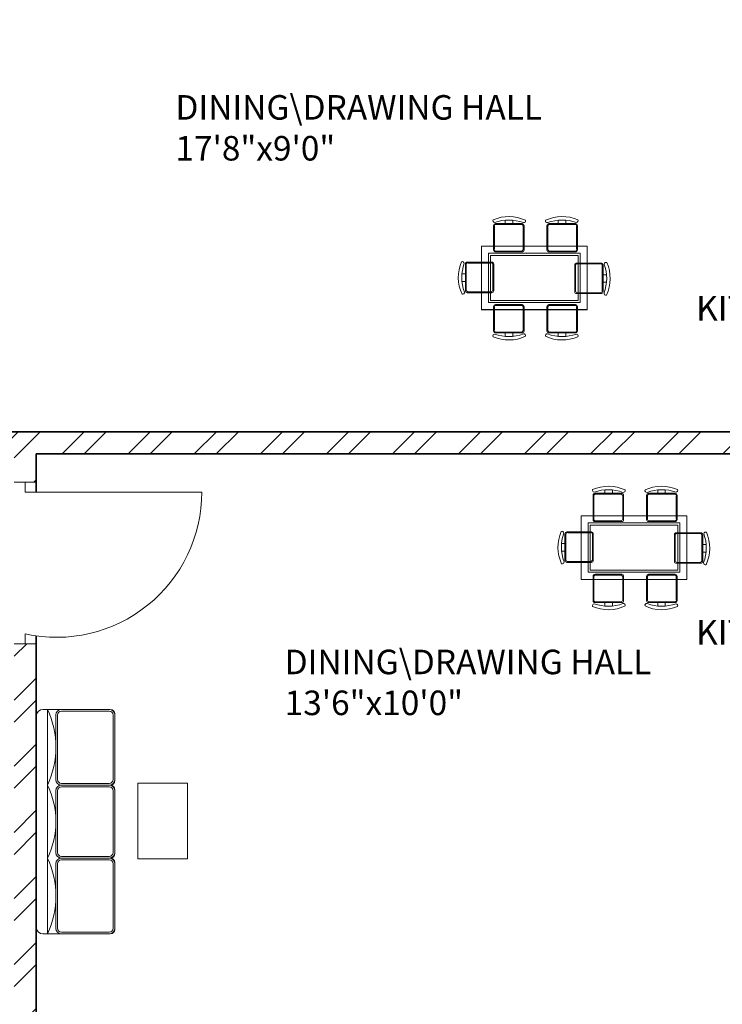
# Model space of a CAD drawing. Units: inches. Extents: x 2165 to 3042, y 1626 to 2968.
# Tile 7 of 11: x 2633 to 2776, y 1990 to 2191. Entities that reach past the tile are written whole.
import ezdxf

# ---------------------------------------------------------------- set-up
doc = ezdxf.new("R2010")
doc.units = ezdxf.units.IN
for name, color, linetype, lineweight in [('A-AREA-IDEN', 7, 'Continuous', 18), ('A-DOOR', 3, 'Continuous', 18), ('A-FURN', 8, 'Continuous', 13), ('A-WALL', 7, 'Continuous', 35), ('A-WALL-PATT', 252, 'Continuous', 13)]:
    doc.layers.add(name, color=color, linetype=linetype, lineweight=lineweight)
doc.styles.get("Standard").update_dxf_attribs({"font": 'arial.ttf'})

# ---------------------------------------------------------------- blocks, each defined once
blk = doc.blocks.new('TABLE-COFFEE')
blk.add_lwpolyline([(0, 15.45), (10.17, 15.45), (10.17, 0), (0, 0)], close=True)
blk = doc.blocks.new('DOOR-36-ENTRY')
for p, q in [((38.25, 32.9), (33.75, 32.9)), ((36, 32.9), (36, 30.9)), ((36, 30.9), (0, 30.9)), ((33.75, 0), (38.25, 0)), ((36, 0), (36, 2))]:
    blk.add_line(p, q)
blk.add_arc((29.6, 30.9), 29.6, 180, 282.4902)

msp = doc.modelspace()

# ---------------------------------------------------------------- hatches: boundary and pattern name
at = {"layer": 'A-WALL-PATT'}
h = msp.add_hatch(dxfattribs=at)
h.set_pattern_fill('ANSI32', color=256)
h.paths.add_polyline_path([(2406.4931, 2332.0783), (2286.6045, 2332.0783), (2286.6045, 2310.967), (2288.8545, 2310.967), (2291.1045, 2310.967), (2291.1045, 2327.5783), (2406.4931, 2327.5783), (2406.4931, 2329.8283)])
h.paths.add_polyline_path([(2439.6045, 2327.5783), (2444.9584, 2327.5783), (2444.9584, 2332.0783), (2430.2901, 2332.0783), (2430.2901, 2329.8283), (2430.2901, 2327.5783), (2435.1045, 2327.5783), (2435.1045, 2219.5783), (2431.0902, 2219.5783), (2431.0902, 2215.0783), (2435.1045, 2215.0783), (2444.1108, 2215.0783), (2444.1108, 2217.3283), (2444.1108, 2219.5783), (2439.6045, 2219.5783)])
h.paths.add_polyline_path([(2497.5418, 2329.8283), (2497.5418, 2332.0783), (2470.1978, 2332.0783), (2470.1978, 2327.5783), (2497.5418, 2327.5783)])
h.paths.add_polyline_path([(2617.9543, 2332.0783), (2557.5418, 2332.0783), (2557.5418, 2327.5783), (2583.6045, 2327.5783), (2583.6045, 2219.5783), (2474.0523, 2219.5783), (2474.0523, 2215.0783), (2583.6045, 2215.0783), (2583.6045, 2107.0783), (2579.3609, 2107.0783), (2579.3609, 2102.5783), (2588.1045, 2102.5783), (2593.5283, 2102.5783), (2593.5283, 2104.8283), (2593.5283, 2107.0783), (2588.1045, 2107.0783), (2588.1045, 2215.0783), (2691.2325, 2215.0783), (2691.2325, 2217.3283), (2691.2325, 2219.5783), (2588.1045, 2219.5783), (2588.1045, 2327.5783), (2617.9543, 2327.5783)])
h.paths.add_polyline_path([(2702.4444, 2329.8283), (2702.4444, 2332.0783), (2677.9543, 2332.0783), (2677.9543, 2327.5783), (2702.4444, 2327.5783)])
h.paths.add_polyline_path([(2736.6045, 2327.5783), (2742.5161, 2327.5783), (2742.5161, 2329.8283), (2742.5161, 2332.0783), (2727.7639, 2332.0783), (2727.7639, 2329.8283), (2727.7639, 2327.5783), (2732.1045, 2327.5783), (2732.1045, 2219.5783), (2726.4404, 2219.5783), (2726.4404, 2215.0783), (2732.1045, 2215.0783), (2742.7291, 2215.0783), (2742.7291, 2217.3283), (2742.7291, 2219.5783), (2736.6045, 2219.5783)])
h.paths.add_polyline_path([(2885.1045, 2332.0783), (2768.4887, 2332.0783), (2768.4887, 2327.5783), (2784.6045, 2327.5783), (2880.6045, 2327.5783), (2880.6045, 2310.967), (2885.1045, 2310.967)])
h.paths.add_polyline_path([(2885.1045, 2250.967), (2880.6045, 2250.967), (2880.6045, 2219.5783), (2776.5755, 2219.5783), (2776.5755, 2215.0783), (2788.1045, 2215.0783), (2788.1045, 2209.8634), (2790.3545, 2209.8634), (2792.6045, 2209.8634), (2792.6045, 2215.0783), (2880.6045, 2215.0783), (2880.6045, 2139.0783), (2871.2037, 2139.0783), (2871.2037, 2134.5783), (2885.1045, 2134.5783)])
h.paths.add_polyline_path([(2545.013, 2107.0783), (2474.0523, 2107.0783), (2291.1045, 2107.0783), (2291.1045, 2102.5783), (2535.6045, 2102.5783), (2535.6045, 2096.8046), (2537.8545, 2096.8046), (2540.1045, 2096.8046), (2540.1045, 2102.5783), (2545.013, 2102.5783), (2545.013, 2104.8283)])
h.paths.add_polyline_path([(2397.7297, 2217.3283), (2397.7297, 2219.5783), (2291.1045, 2219.5783), (2291.1045, 2250.967), (2286.6045, 2250.967), (2286.6045, 2206.1346), (2288.8545, 2206.1346), (2291.1045, 2206.1346), (2291.1045, 2215.0783), (2367.1045, 2215.0783), (2367.1045, 2212.2868), (2371.6045, 2212.2868), (2371.6045, 2215.0783), (2397.7297, 2215.0783)])
h.paths.add_polyline_path([(2291.1045, 1978.5783), (2367.1045, 1978.5783), (2371.6045, 1978.5783), (2373.2641, 1978.5783), (2374.4883, 1978.5783), (2374.4883, 1980.8283), (2374.4883, 1983.0783), (2371.6045, 1983.0783), (2371.6045, 1986.964), (2369.9051, 1986.964), (2369.3545, 1986.964), (2367.1045, 1986.964), (2367.1045, 1983.0783), (2291.1045, 1983.0783), (2291.1045, 2001.1808), (2286.6045, 2001.1808), (2286.6045, 1947.0203), (2288.8545, 1947.0203), (2291.1045, 1947.0203)])
h.paths.add_polyline_path([(2291.1045, 1887.0203), (2286.6045, 1887.0203), (2286.6045, 1842.0783), (2381.2561, 1842.0783), (2381.2561, 1844.3283), (2381.2561, 1846.5783), (2363.1045, 1846.5783), (2291.1045, 1846.5783)])
h.paths.add_polyline_path([(2415.6045, 1978.5783), (2421.1681, 1978.5783), (2421.1681, 1983.0783), (2415.6045, 1983.0783), (2406.5227, 1983.0783), (2406.5227, 1980.8283), (2406.5227, 1978.5783), (2411.1045, 1978.5783), (2411.1045, 1846.5783), (2406.7549, 1846.5783), (2406.7549, 1842.0783), (2419.2885, 1842.0783), (2419.2885, 1844.3283), (2419.2885, 1846.5783), (2415.6045, 1846.5783)])
h.paths.add_polyline_path([(2586.6045, 1982.779), (2586.6045, 1991.5911), (2582.1045, 1991.5911), (2582.1045, 1982.779), (2540.1045, 1982.779), (2540.1045, 2036.779), (2582.1045, 2036.779), (2582.1045, 2027.6051), (2586.6045, 2027.6051), (2586.6045, 2041.279), (2582.1045, 2041.279), (2540.1045, 2041.279), (2540.1045, 2063.9064), (2537.8545, 2063.9064), (2535.6045, 2063.9064), (2535.6045, 1983.0783), (2455.068, 1983.0783), (2455.068, 1978.5783), (2535.6045, 1978.5783), (2535.6045, 1846.5783), (2522.622, 1846.5783), (2522.622, 1842.0783), (2535.6045, 1842.0783), (2535.6045, 1806.0783), (2535.6045, 1801.5783), (2556.726, 1801.5783), (2556.726, 1803.8283), (2556.726, 1806.0783), (2540.1045, 1806.0783), (2540.1045, 1842.0783), (2540.1045, 1846.5783), (2540.1045, 1978.279), (2586.6045, 1978.279)])
h.paths.add_polyline_path([(2636.1045, 1978.5783), (2717.6642, 1978.5783), (2717.6642, 1980.8283), (2717.6642, 1983.0783), (2636.1045, 1983.0783), (2636.1045, 2063.9064), (2633.8545, 2063.9064), (2631.6045, 2063.9064), (2631.6045, 1846.5783), (2631.6045, 1842.0783), (2631.6045, 1806.0783), (2604.726, 1806.0783), (2604.726, 1801.5783), (2636.1045, 1801.5783), (2636.1045, 1842.0783), (2644.3411, 1842.0783), (2644.3411, 1844.3283), (2644.3411, 1846.5783), (2636.1045, 1846.5783)])
h.paths.add_polyline_path([(2760.6045, 1978.5783), (2764.9931, 1978.5783), (2764.9931, 1983.0783), (2750.4727, 1983.0783), (2750.4727, 1980.8283), (2750.4727, 1978.5783), (2756.1045, 1978.5783), (2756.1045, 1846.5783), (2749.4543, 1846.5783), (2749.4543, 1842.0783), (2765.1894, 1842.0783), (2765.1894, 1846.5783), (2760.6045, 1846.5783)])
h.paths.add_polyline_path([(2880.6045, 1983.0783), (2804.6045, 1983.0783), (2804.6045, 1988.3825), (2802.3545, 1988.3825), (2800.1045, 1988.3825), (2800.1045, 1983.0783), (2800.1045, 1978.5783), (2880.6045, 1978.5783)])
h.paths.add_polyline_path([(2885.1045, 2075.5783), (2871.2037, 2075.5783), (2871.2037, 2071.0783), (2880.6045, 2071.0783), (2880.6045, 1948.8144), (2885.1045, 1948.8144)])
h.paths.add_polyline_path([(2885.1045, 1888.8144), (2880.6045, 1888.8144), (2880.6045, 1846.5783), (2792.1167, 1846.5783), (2792.1167, 1842.0783), (2885.1045, 1842.0783)])
h.paths.add_polyline_path([(2724.4848, 1846.5783), (2708.1045, 1846.5783), (2692.3411, 1846.5783), (2692.3411, 1842.0783), (2724.4848, 1842.0783), (2724.4848, 1844.3283)])
h.paths.add_polyline_path([(2474.622, 1844.4672), (2474.622, 1846.5783), (2444.7417, 1846.5783), (2444.7417, 1842.0783), (2474.622, 1842.0783)])
h = msp.add_hatch(dxfattribs=at)
h.set_pattern_fill('ANSI32', color=256)
h.paths.add_polyline_path([(2834.3545, 2109.2607), (2832.1045, 2109.2607), (2829.8545, 2109.2607), (2829.8545, 2107.0783), (2788.1045, 2107.0783), (2627.8367, 2107.0783), (2627.8367, 2102.5783), (2631.6045, 2102.5783), (2631.6045, 2096.8046), (2636.1045, 2096.8046), (2636.1045, 2102.5783), (2788.1045, 2102.5783), (2829.8545, 2102.5783), (2829.8545, 2099.5599), (2834.3545, 2099.5599), (2834.3545, 2102.5783)])
h.paths.add_polyline_path([(2834.3545, 2162.7002), (2834.3545, 2167.2002), (2792.6045, 2167.2002), (2792.6045, 2188.8893), (2790.3545, 2188.8893), (2788.1045, 2188.8893), (2788.1045, 2162.7002), (2829.8545, 2162.7002), (2829.8545, 2134.5783), (2829.8545, 2129.9534), (2834.3545, 2129.9534), (2834.3545, 2134.5783), (2847.2037, 2134.5783), (2847.2037, 2139.0783), (2834.3545, 2139.0783)])
h.paths.add_polyline_path([(2834.3545, 2071.0783), (2847.2037, 2071.0783), (2847.2037, 2075.5783), (2834.3545, 2075.5783), (2834.3545, 2078.8214), (2829.8545, 2078.8214), (2829.8545, 2075.5783), (2829.8545, 2034.1177), (2800.1045, 2034.1177), (2800.1045, 2011.8162), (2802.3375, 2011.8162), (2804.6045, 2011.8162), (2804.6045, 2029.6177), (2834.3545, 2029.6177), (2834.3545, 2034.1177)])

# ---------------------------------------------------------------- linework, layer by layer
at = {"layer": 'A-DOOR'}
for p, q in [((2636.1045, 2096.8046), (2633.8545, 2096.8046)), ((2636.1045, 2063.9064), (2633.8545, 2063.9064))]:
    msp.add_line(p, q, dxfattribs=at)
at = {"layer": 'A-FURN'}
for points in [[(2729.5671, 2149.7833, -0.17580919), (2735.4417, 2149.7388, 0.57839206), (2735.8868, 2150.2282, 0.21452438), (2729.2556, 2150.3172, 0.55201397), (2729.5671, 2149.7833, -0.06507904)], [(2729.5672, 2149.7831, -0.17580919), (2735.4417, 2149.7386, 0.57839206), (2735.8868, 2150.228, 0.21452438), (2729.2556, 2150.3169, 0.55201397), (2729.5672, 2149.7831, -0.06507904)], [(2733.2769, 2149.5475), (2733.2769, 2150.2373, -0.06475861)], [(2733.2769, 2149.5473), (2733.2769, 2150.237, -0.06475861)], [(2740.3874, 2149.7388, -0.57839206), (2739.9423, 2150.2282, -0.21452438), (2746.5735, 2150.3172, -0.55201397), (2746.2619, 2149.7833, 0.1758092), (2740.3874, 2149.7388)], [(2740.3874, 2149.7386, -0.57839206), (2739.9423, 2150.228, -0.21452438), (2746.5735, 2150.3169, -0.55201397), (2746.2619, 2149.7831, 0.1758092), (2740.3874, 2149.7386)], [(2742.5522, 2149.5475), (2742.5522, 2150.2373, 0.06475861)], [(2742.5522, 2149.5473), (2742.5522, 2150.237, 0.06475861)], [(2735.1925, 2149.5475), (2729.7387, 2149.5475, 0.41421356), (2729.3572, 2149.166), (2729.3572, 2144.1514, 0.41421356), (2729.7387, 2143.7698), (2735.1925, 2143.7698, 0.41421356), (2735.574, 2144.1514), (2735.574, 2149.166, 0.41421356), (2735.1925, 2149.5475)], [(2735.1925, 2149.5473), (2729.7387, 2149.5473, 0.41421356), (2729.3572, 2149.1658), (2729.3572, 2144.1511, 0.41421356), (2729.7387, 2143.7696), (2735.1925, 2143.7696, 0.41421356), (2735.574, 2144.1511), (2735.574, 2149.1658, 0.41421356), (2735.1925, 2149.5473)], [(2746.0904, 2149.5475, -0.41421356), (2746.4719, 2149.166), (2746.4719, 2144.1514, -0.41421356), (2746.0904, 2143.7698), (2740.6366, 2143.7698, -0.41421356), (2740.255, 2144.1514), (2740.255, 2149.166, -0.41421356), (2740.6366, 2149.5475), (2746.0904, 2149.5475)], [(2746.0904, 2149.5473, -0.41421356), (2746.4719, 2149.1658), (2746.4719, 2144.1511, -0.41421356), (2746.0904, 2143.7696), (2740.6366, 2143.7696, -0.41421356), (2740.2551, 2144.1511), (2740.2551, 2149.1658, -0.41421356), (2740.6366, 2149.5473), (2746.0904, 2149.5473)], [(2723.4212, 2135.5971, -0.57839206), (2722.9318, 2135.152, -0.21452438), (2722.8429, 2141.7832, -0.55201397), (2723.3767, 2141.4717, 0.17580937), (2723.4212, 2135.5971)], [(2723.4212, 2135.5969, -0.57839206), (2722.9319, 2135.1518, -0.21452438), (2722.8429, 2141.783, -0.55201397), (2723.3767, 2141.4714, 0.17580937), (2723.4212, 2135.5969)], [(2723.6125, 2141.3001, -0.41421356), (2723.994, 2141.6816), (2729.0087, 2141.6816, -0.41421356), (2729.3902, 2141.3001), (2729.3902, 2135.8463, -0.41421356), (2729.0087, 2135.4648), (2723.994, 2135.4648, -0.41421356), (2723.6125, 2135.8463), (2723.6125, 2141.3001)], [(2723.6125, 2141.2999, -0.41421356), (2723.9941, 2141.6814), (2729.0087, 2141.6814, -0.41421356), (2729.3902, 2141.2999), (2729.3902, 2135.8461, -0.41421356), (2729.0087, 2135.4645), (2723.9941, 2135.4645, -0.41421356), (2723.6125, 2135.8461), (2723.6125, 2141.2999)], [(2751.6968, 2141.1133, 0.41421356), (2751.3153, 2141.4949), (2746.3006, 2141.4949, 0.41421356), (2745.9191, 2141.1133), (2745.9191, 2135.6595, 0.41421356), (2746.3006, 2135.278), (2751.3153, 2135.278, 0.41421356), (2751.6968, 2135.6595), (2751.6968, 2141.1133)], [(2751.6968, 2141.1131, 0.41421356), (2751.3153, 2141.4946), (2746.3006, 2141.4946, 0.41421356), (2745.9191, 2141.1131), (2745.9191, 2135.6593, 0.41421356), (2746.3006, 2135.2778), (2751.3153, 2135.2778, 0.41421356), (2751.6968, 2135.6593), (2751.6968, 2141.1131)], [(2751.9326, 2141.2849, -0.17580919), (2751.8881, 2135.4103, 0.57839206), (2752.3775, 2134.9653, 0.21452438), (2752.4664, 2141.5964, 0.55201397), (2751.9326, 2141.2849, -0.06507904)], [(2751.9326, 2141.2847, -0.17580919), (2751.8881, 2135.4101, 0.57839206), (2752.3775, 2134.965, 0.21452438), (2752.4664, 2141.5962, 0.55201397), (2751.9326, 2141.2847, -0.06507904)], [(2723.6125, 2137.762), (2722.9228, 2137.762, 0.06475861)], [(2723.6125, 2137.7617), (2722.9228, 2137.7617, 0.06475861)], [(2751.6968, 2137.5752), (2752.3865, 2137.5752, -0.06475861)], [(2751.6968, 2137.575), (2752.3866, 2137.575, -0.06475861)], [(2735.1925, 2127.2563), (2729.7387, 2127.2563, -0.41421356), (2729.3572, 2127.6378), (2729.3572, 2132.6525, -0.41421356), (2729.7387, 2133.034), (2735.1925, 2133.034, -0.41421356), (2735.574, 2132.6525), (2735.574, 2127.6378, -0.41421356), (2735.1925, 2127.2563)], [(2735.1925, 2127.2561), (2729.7387, 2127.2561, -0.41421356), (2729.3572, 2127.6376), (2729.3572, 2132.6522, -0.41421356), (2729.7387, 2133.0338), (2735.1925, 2133.0338, -0.41421356), (2735.574, 2132.6522), (2735.574, 2127.6376, -0.41421356), (2735.1925, 2127.2561)], [(2746.0904, 2127.2563, 0.41421356), (2746.4719, 2127.6378), (2746.4719, 2132.6525, 0.41421356), (2746.0904, 2133.034), (2740.6366, 2133.034, 0.41421356), (2740.255, 2132.6525), (2740.255, 2127.6378, 0.41421356), (2740.6366, 2127.2563), (2746.0904, 2127.2563)], [(2746.0904, 2127.2561, 0.41421356), (2746.4719, 2127.6376), (2746.4719, 2132.6522, 0.41421356), (2746.0904, 2133.0338), (2740.6366, 2133.0338, 0.41421356), (2740.2551, 2132.6522), (2740.2551, 2127.6376, 0.41421356), (2740.6366, 2127.2561), (2746.0904, 2127.2561)], [(2735.4417, 2127.065, -0.57839206), (2735.8868, 2126.5756, -0.21452438), (2729.2556, 2126.4867, -0.55201397), (2729.5671, 2127.0205, 0.17580929), (2735.4417, 2127.065)], [(2735.4417, 2127.0648, -0.57839206), (2735.8868, 2126.5754, -0.21452438), (2729.2556, 2126.4864, -0.55201397), (2729.5672, 2127.0203, 0.17580929), (2735.4417, 2127.0648)], [(2733.2769, 2127.2563), (2733.2769, 2126.5666, 0.06475861)], [(2733.2769, 2127.2561), (2733.2769, 2126.5663, 0.06475861)], [(2746.2619, 2127.0205, -0.17580928), (2740.3874, 2127.065, 0.57839206), (2739.9423, 2126.5756, 0.21452438), (2746.5735, 2126.4867, 0.55201397), (2746.2619, 2127.0205, -0.06507904)], [(2746.2619, 2127.0203, -0.17580928), (2740.3874, 2127.0648, 0.57839206), (2739.9423, 2126.5754, 0.21452438), (2746.5735, 2126.4864, 0.55201397), (2746.2619, 2127.0203, -0.06507904)], [(2742.5522, 2127.2563), (2742.5522, 2126.5666, -0.06475861)], [(2742.5522, 2127.2561), (2742.5522, 2126.5663, -0.06475861)], [(2749.8774, 2094.8015, -0.17580919), (2755.752, 2094.757, 0.57839206), (2756.197, 2095.2464, 0.21452438), (2749.5659, 2095.3354, 0.55201397), (2749.8774, 2094.8015, -0.06507904)], [(2749.8774, 2094.8013, -0.17580919), (2755.752, 2094.7568, 0.57839206), (2756.197, 2095.2462, 0.21452438), (2749.5659, 2095.3351, 0.55201397), (2749.8774, 2094.8013, -0.06507904)], [(2760.6976, 2094.757, -0.57839206), (2760.2526, 2095.2464, -0.21452438), (2766.8837, 2095.3354, -0.55201397), (2766.5722, 2094.8015, 0.1758092), (2760.6976, 2094.757)], [(2760.6976, 2094.7568, -0.57839206), (2760.2526, 2095.2462, -0.21452438), (2766.8837, 2095.3351, -0.55201397), (2766.5722, 2094.8013, 0.1758092), (2760.6976, 2094.7568)], [(2755.5027, 2094.5657), (2750.049, 2094.5657, 0.41421356), (2749.6674, 2094.1842), (2749.6674, 2089.1696, 0.41421356), (2750.049, 2088.788), (2755.5027, 2088.788, 0.41421356), (2755.8843, 2089.1696), (2755.8843, 2094.1842, 0.41421356), (2755.5027, 2094.5657)], [(2755.5027, 2094.5655), (2750.049, 2094.5655, 0.41421356), (2749.6674, 2094.184), (2749.6674, 2089.1693, 0.41421356), (2750.049, 2088.7878), (2755.5027, 2088.7878, 0.41421356), (2755.8843, 2089.1693), (2755.8843, 2094.184, 0.41421356), (2755.5027, 2094.5655)], [(2753.5871, 2094.5657), (2753.5871, 2095.2555, -0.06475861)], [(2753.5871, 2094.5655), (2753.5871, 2095.2553, -0.06475861)], [(2766.4006, 2094.5657, -0.41421356), (2766.7821, 2094.1842), (2766.7821, 2089.1696, -0.41421356), (2766.4006, 2088.788), (2760.9468, 2088.788, -0.41421356), (2760.5653, 2089.1696), (2760.5653, 2094.1842, -0.41421356), (2760.9468, 2094.5657), (2766.4006, 2094.5657)], [(2766.4006, 2094.5655, -0.41421356), (2766.7822, 2094.184), (2766.7822, 2089.1693, -0.41421356), (2766.4006, 2088.7878), (2760.9468, 2088.7878, -0.41421356), (2760.5653, 2089.1693), (2760.5653, 2094.184, -0.41421356), (2760.9468, 2094.5655), (2766.4006, 2094.5655)], [(2762.8625, 2094.5657), (2762.8625, 2095.2555, 0.06475861)], [(2762.8625, 2094.5655), (2762.8625, 2095.2553, 0.06475861)], [(2743.7314, 2080.6153, -0.57839206), (2743.2421, 2080.1703, -0.21452438), (2743.1531, 2086.8014, -0.55201397), (2743.687, 2086.4899, 0.17580937), (2743.7314, 2080.6153)], [(2743.7315, 2080.6151, -0.57839206), (2743.2421, 2080.17, -0.21452438), (2743.1531, 2086.8012, -0.55201397), (2743.687, 2086.4897, 0.17580937), (2743.7315, 2080.6151)], [(2743.9227, 2086.3183, -0.41421356), (2744.3043, 2086.6999), (2749.3189, 2086.6999, -0.41421356), (2749.7005, 2086.3183), (2749.7005, 2080.8645, -0.41421356), (2749.3189, 2080.483), (2744.3043, 2080.483, -0.41421356), (2743.9227, 2080.8645), (2743.9227, 2086.3183)], [(2743.9228, 2086.3181, -0.41421356), (2744.3043, 2086.6996), (2749.3189, 2086.6996, -0.41421356), (2749.7005, 2086.3181), (2749.7005, 2080.8643, -0.41421356), (2749.3189, 2080.4828), (2744.3043, 2080.4828, -0.41421356), (2743.9228, 2080.8643), (2743.9228, 2086.3181)], [(2772.0071, 2086.1315, 0.41421356), (2771.6255, 2086.5131), (2766.6109, 2086.5131, 0.41421356), (2766.2293, 2086.1315), (2766.2293, 2080.6778, 0.41421356), (2766.6109, 2080.2962), (2771.6255, 2080.2962, 0.41421356), (2772.0071, 2080.6778), (2772.0071, 2086.1315)], [(2772.0071, 2086.1313, 0.41421356), (2771.6255, 2086.5128), (2766.6109, 2086.5128, 0.41421356), (2766.2293, 2086.1313), (2766.2293, 2080.6775, 0.41421356), (2766.6109, 2080.296), (2771.6255, 2080.296, 0.41421356), (2772.0071, 2080.6775), (2772.0071, 2086.1313)], [(2772.2428, 2086.3031, -0.17580919), (2772.1983, 2080.4285, 0.57839206), (2772.6877, 2079.9835, 0.21452438), (2772.7767, 2086.6146, 0.55201397), (2772.2428, 2086.3031, -0.06507904)], [(2772.2428, 2086.3029, -0.17580919), (2772.1984, 2080.4283, 0.57839206), (2772.6877, 2079.9833, 0.21452438), (2772.7767, 2086.6144, 0.55201397), (2772.2428, 2086.3029, -0.06507904)], [(2743.9227, 2082.7802), (2743.233, 2082.7802, 0.06475861)], [(2743.9228, 2082.7799), (2743.233, 2082.7799, 0.06475861)], [(2772.0071, 2082.5934), (2772.6968, 2082.5934, -0.06475861)], [(2772.0071, 2082.5932), (2772.6968, 2082.5932, -0.06475861)], [(2755.5027, 2072.2745), (2750.049, 2072.2745, -0.41421356), (2749.6674, 2072.6561), (2749.6674, 2077.6707, -0.41421356), (2750.049, 2078.0522), (2755.5027, 2078.0522, -0.41421356), (2755.8843, 2077.6707), (2755.8843, 2072.6561, -0.41421356), (2755.5027, 2072.2745)], [(2755.5027, 2072.2743), (2750.049, 2072.2743, -0.41421356), (2749.6674, 2072.6558), (2749.6674, 2077.6705, -0.41421356), (2750.049, 2078.052), (2755.5027, 2078.052, -0.41421356), (2755.8843, 2077.6705), (2755.8843, 2072.6558, -0.41421356), (2755.5027, 2072.2743)], [(2766.4006, 2072.2745, 0.41421356), (2766.7821, 2072.6561), (2766.7821, 2077.6707, 0.41421356), (2766.4006, 2078.0522), (2760.9468, 2078.0522, 0.41421356), (2760.5653, 2077.6707), (2760.5653, 2072.6561, 0.41421356), (2760.9468, 2072.2745), (2766.4006, 2072.2745)], [(2766.4006, 2072.2743, 0.41421356), (2766.7822, 2072.6558), (2766.7822, 2077.6705, 0.41421356), (2766.4006, 2078.052), (2760.9468, 2078.052, 0.41421356), (2760.5653, 2077.6705), (2760.5653, 2072.6558, 0.41421356), (2760.9468, 2072.2743), (2766.4006, 2072.2743)], [(2755.752, 2072.0832, -0.57839206), (2756.197, 2071.5938, -0.21452438), (2749.5659, 2071.5049, -0.55201397), (2749.8774, 2072.0387, 0.17580929), (2755.752, 2072.0832)], [(2755.752, 2072.083, -0.57839206), (2756.197, 2071.5936, -0.21452438), (2749.5659, 2071.5046, -0.55201397), (2749.8774, 2072.0385, 0.17580929), (2755.752, 2072.083)], [(2753.5871, 2072.2745), (2753.5871, 2071.5848, 0.06475861)], [(2753.5871, 2072.2743), (2753.5871, 2071.5845, 0.06475861)], [(2766.5722, 2072.0387, -0.17580928), (2760.6976, 2072.0832, 0.57839206), (2760.2526, 2071.5938, 0.21452438), (2766.8837, 2071.5049, 0.55201397), (2766.5722, 2072.0387, -0.06507904)], [(2766.5722, 2072.0385, -0.17580928), (2760.6976, 2072.083, 0.57839206), (2760.2526, 2071.5936, 0.21452438), (2766.8837, 2071.5046, 0.55201397), (2766.5722, 2072.0385, -0.06507904)], [(2762.8625, 2072.2745), (2762.8625, 2071.5848, -0.06475861)], [(2762.8625, 2072.2743), (2762.8625, 2071.5845, -0.06475861)]]:
    msp.add_lwpolyline(points, format="xyb", dxfattribs=at)
for points in [[(2731.7503, 2150.2498), (2731.7503, 2149.5475)], [(2731.7503, 2150.2496), (2731.7503, 2149.5473)], [(2744.0788, 2150.2498), (2744.0788, 2149.5475)], [(2744.0788, 2150.2496), (2744.0788, 2149.5473)], [(2722.9102, 2139.2885), (2723.6125, 2139.2885)], [(2722.9102, 2139.2883), (2723.6125, 2139.2883)], [(2752.3991, 2139.1018), (2751.6968, 2139.1018)], [(2752.3991, 2139.1015), (2751.6968, 2139.1015)], [(2731.7503, 2126.554), (2731.7503, 2127.2563)], [(2731.7503, 2126.5538), (2731.7503, 2127.2561)], [(2744.0788, 2126.554), (2744.0788, 2127.2563)], [(2744.0788, 2126.5538), (2744.0788, 2127.2561)], [(2752.0605, 2095.268), (2752.0605, 2094.5657)], [(2752.0605, 2095.2678), (2752.0605, 2094.5655)], [(2764.3891, 2095.268), (2764.3891, 2094.5657)], [(2764.3891, 2095.2678), (2764.3891, 2094.5655)], [(2743.2205, 2084.3068), (2743.9227, 2084.3068)], [(2743.2205, 2084.3065), (2743.9228, 2084.3065)], [(2772.7093, 2084.12), (2772.0071, 2084.12)], [(2772.7093, 2084.1198), (2772.0071, 2084.1198)], [(2752.0605, 2071.5722), (2752.0605, 2072.2745)], [(2752.0605, 2071.572), (2752.0605, 2072.2743)], [(2764.3891, 2071.5722), (2764.3891, 2072.2745)], [(2764.3891, 2071.572), (2764.3891, 2072.2743)], [(2638.3929, 2050.512), (2638.3929, 2004.743)]]:
    msp.add_lwpolyline(points, dxfattribs=at)
for points in [[(2729.741, 2149.3756), (2735.0206, 2149.3756, -0.41421356), (2735.4021, 2148.9941), (2735.4021, 2144.3232, -0.41421356), (2735.0206, 2143.9417), (2729.741, 2143.9417, -0.51206948), (2729.5291, 2144.3232), (2729.5291, 2148.9941, -0.51206948)], [(2729.7411, 2149.3754), (2735.0206, 2149.3754, -0.41421356), (2735.4022, 2148.9939), (2735.4022, 2144.323, -0.41421356), (2735.0206, 2143.9415), (2729.7411, 2143.9415, -0.51206948), (2729.5291, 2144.323), (2729.5291, 2148.9939, -0.51206948)], [(2746.088, 2149.3756), (2740.8085, 2149.3756, 0.41421356), (2740.4269, 2148.9941), (2740.4269, 2144.3232, 0.41421356), (2740.8085, 2143.9417), (2746.088, 2143.9417, 0.51206948), (2746.3, 2144.3232), (2746.3, 2148.9941, 0.51206948)], [(2746.088, 2149.3754), (2740.8085, 2149.3754, 0.41421356), (2740.4269, 2148.9939), (2740.4269, 2144.323, 0.41421356), (2740.8085, 2143.9415), (2746.088, 2143.9415, 0.51206948), (2746.3, 2144.323), (2746.3, 2148.9939, 0.51206948)], [(2723.7844, 2141.2978), (2723.7844, 2136.0182, 0.41421356), (2724.1659, 2135.6367), (2728.8368, 2135.6367, 0.41421356), (2729.2183, 2136.0182), (2729.2183, 2141.2978, 0.51206948), (2728.8368, 2141.5097), (2724.1659, 2141.5097, 0.51206948)], [(2723.7844, 2141.2975), (2723.7844, 2136.018, 0.41421356), (2724.166, 2135.6364), (2728.8368, 2135.6364, 0.41421356), (2729.2183, 2136.018), (2729.2183, 2141.2975, 0.51206948), (2728.8368, 2141.5095), (2724.166, 2141.5095, 0.51206948)], [(2751.5249, 2141.111), (2751.5249, 2135.8314, -0.41421356), (2751.1434, 2135.4499), (2746.4725, 2135.4499, -0.41421356), (2746.091, 2135.8314), (2746.091, 2141.111, -0.51206948), (2746.4725, 2141.323), (2751.1434, 2141.323, -0.51206948)], [(2751.5249, 2141.1108), (2751.5249, 2135.8312, -0.41421356), (2751.1434, 2135.4497), (2746.4725, 2135.4497, -0.41421356), (2746.091, 2135.8312), (2746.091, 2141.1108, -0.51206948), (2746.4725, 2141.3227), (2751.1434, 2141.3227, -0.51206948)], [(2729.741, 2127.4282), (2735.0206, 2127.4282, 0.41421356), (2735.4021, 2127.8097), (2735.4021, 2132.4806, 0.41421356), (2735.0206, 2132.8621), (2729.741, 2132.8621, 0.51206948), (2729.5291, 2132.4806), (2729.5291, 2127.8097, 0.51206948)], [(2729.7411, 2127.4279), (2735.0206, 2127.4279, 0.41421356), (2735.4022, 2127.8095), (2735.4022, 2132.4803, 0.41421356), (2735.0206, 2132.8619), (2729.7411, 2132.8619, 0.51206948), (2729.5291, 2132.4803), (2729.5291, 2127.8095, 0.51206948)], [(2746.088, 2127.4282), (2740.8085, 2127.4282, -0.41421356), (2740.4269, 2127.8097), (2740.4269, 2132.4806, -0.41421356), (2740.8085, 2132.8621), (2746.088, 2132.8621, -0.51206948), (2746.3, 2132.4806), (2746.3, 2127.8097, -0.51206948)], [(2746.088, 2127.4279), (2740.8085, 2127.4279, -0.41421356), (2740.4269, 2127.8095), (2740.4269, 2132.4803, -0.41421356), (2740.8085, 2132.8619), (2746.088, 2132.8619, -0.51206948), (2746.3, 2132.4803), (2746.3, 2127.8095, -0.51206948)], [(2750.0513, 2094.3939), (2755.3308, 2094.3939, -0.41421356), (2755.7124, 2094.0123), (2755.7124, 2089.3415, -0.41421356), (2755.3308, 2088.9599), (2750.0513, 2088.9599, -0.51206948), (2749.8393, 2089.3415), (2749.8393, 2094.0123, -0.51206948)], [(2750.0513, 2094.3936), (2755.3309, 2094.3936, -0.41421356), (2755.7124, 2094.0121), (2755.7124, 2089.3412, -0.41421356), (2755.3309, 2088.9597), (2750.0513, 2088.9597, -0.51206948), (2749.8393, 2089.3412), (2749.8393, 2094.0121, -0.51206948)], [(2766.3983, 2094.3939), (2761.1187, 2094.3939, 0.41421356), (2760.7372, 2094.0123), (2760.7372, 2089.3415, 0.41421356), (2761.1187, 2088.9599), (2766.3983, 2088.9599, 0.51206948), (2766.6103, 2089.3415), (2766.6103, 2094.0123, 0.51206948)], [(2766.3983, 2094.3936), (2761.1187, 2094.3936, 0.41421356), (2760.7372, 2094.0121), (2760.7372, 2089.3412, 0.41421356), (2761.1187, 2088.9597), (2766.3983, 2088.9597, 0.51206948), (2766.6103, 2089.3412), (2766.6103, 2094.0121, 0.51206948)], [(2744.0946, 2086.316), (2744.0946, 2081.0364, 0.41421356), (2744.4762, 2080.6549), (2749.147, 2080.6549, 0.41421356), (2749.5286, 2081.0364), (2749.5286, 2086.316, 0.51206948), (2749.147, 2086.528), (2744.4762, 2086.528, 0.51206948)], [(2744.0946, 2086.3158), (2744.0946, 2081.0362, 0.41421356), (2744.4762, 2080.6547), (2749.147, 2080.6547, 0.41421356), (2749.5286, 2081.0362), (2749.5286, 2086.3158, 0.51206948), (2749.147, 2086.5277), (2744.4762, 2086.5277, 0.51206948)], [(2771.8352, 2086.1292), (2771.8352, 2080.8497, -0.41421356), (2771.4536, 2080.4681), (2766.7828, 2080.4681, -0.41421356), (2766.4012, 2080.8497), (2766.4012, 2086.1292, -0.51206948), (2766.7828, 2086.3412), (2771.4536, 2086.3412, -0.51206948)], [(2771.8352, 2086.129), (2771.8352, 2080.8494, -0.41421356), (2771.4536, 2080.4679), (2766.7828, 2080.4679, -0.41421356), (2766.4012, 2080.8494), (2766.4012, 2086.129, -0.51206948), (2766.7828, 2086.341), (2771.4536, 2086.341, -0.51206948)], [(2750.0513, 2072.4464), (2755.3308, 2072.4464, 0.41421356), (2755.7124, 2072.8279), (2755.7124, 2077.4988, 0.41421356), (2755.3308, 2077.8803), (2750.0513, 2077.8803, 0.51206948), (2749.8393, 2077.4988), (2749.8393, 2072.8279, 0.51206948)], [(2750.0513, 2072.4462), (2755.3309, 2072.4462, 0.41421356), (2755.7124, 2072.8277), (2755.7124, 2077.4986, 0.41421356), (2755.3309, 2077.8801), (2750.0513, 2077.8801, 0.51206948), (2749.8393, 2077.4986), (2749.8393, 2072.8277, 0.51206948)], [(2766.3983, 2072.4464), (2761.1187, 2072.4464, -0.41421356), (2760.7372, 2072.8279), (2760.7372, 2077.4988, -0.41421356), (2761.1187, 2077.8803), (2766.3983, 2077.8803, -0.51206948), (2766.6103, 2077.4988), (2766.6103, 2072.8279, -0.51206948)], [(2766.3983, 2072.4462), (2761.1187, 2072.4462, -0.41421356), (2760.7372, 2072.8277), (2760.7372, 2077.4986, -0.41421356), (2761.1187, 2077.8801), (2766.3983, 2077.8801, -0.51206948), (2766.6103, 2077.4986), (2766.6103, 2072.8277, -0.51206948)], [(2650.9794, 2050.512), (2641.2535, 2050.512, 0.41421356), (2640.1092, 2049.3678), (2640.1092, 2036.2092, 0.41421356), (2641.2535, 2035.065), (2650.9794, 2035.065, 0.41421356), (2652.1236, 2036.2092), (2652.1236, 2049.3678, 0.41421356)], [(2650.9794, 2050.1687), (2641.2535, 2050.1687, 0.41421356), (2640.4525, 2049.3678), (2640.4525, 2036.2092, 0.41421356), (2641.2535, 2035.4082), (2650.9794, 2035.4082, 0.41421356), (2651.7803, 2036.2092), (2651.7803, 2049.3678, 0.41421356)], [(2650.9794, 2020.1901), (2641.2535, 2020.1901, -0.41421356), (2640.1092, 2021.3343), (2640.1092, 2033.9207, -0.41421356), (2641.2535, 2035.065), (2650.9794, 2035.065, -0.41421356), (2652.1236, 2033.9207), (2652.1236, 2021.3343, -0.41421356)], [(2650.9794, 2020.5333), (2641.2535, 2020.5333, -0.41421356), (2640.4525, 2021.3343), (2640.4525, 2033.9207, -0.41421356), (2641.2535, 2034.7217), (2650.9794, 2034.7217, -0.41421356), (2651.7803, 2033.9207), (2651.7803, 2021.3343, -0.41421356)], [(2650.9794, 2020.1901), (2641.2535, 2020.1901, 0.41421356), (2640.1092, 2019.0458), (2640.1092, 2005.8873, 0.41421356), (2641.2535, 2004.743), (2650.9794, 2004.743, 0.41421356), (2652.1236, 2005.8873), (2652.1236, 2019.0458, 0.41421356)], [(2650.9794, 2019.8468), (2641.2535, 2019.8468, 0.41421356), (2640.4525, 2019.0458), (2640.4525, 2005.8873, 0.41421356), (2641.2535, 2005.0863), (2650.9794, 2005.0863, 0.41421356), (2651.7803, 2005.8873), (2651.7803, 2019.0458, 0.41421356)]]:
    msp.add_lwpolyline(points, format="xyb", close=True, dxfattribs=at)
for points in [[(2726.8994, 2144.9417), (2748.4676, 2144.9417), (2748.4676, 2132.0007), (2726.8994, 2132.0007)], [(2726.8994, 2144.9415), (2748.4676, 2144.9415), (2748.4676, 2132.0005), (2726.8994, 2132.0005)], [(2728.3373, 2143.5038), (2747.0297, 2143.5038), (2747.0297, 2133.4386), (2728.3373, 2133.4386)], [(2728.3373, 2143.5036), (2747.0298, 2143.5036), (2747.0298, 2133.4384), (2728.3373, 2133.4384)], [(2728.7686, 2143.0724), (2746.5984, 2143.0724), (2746.5984, 2133.87), (2728.7686, 2133.87)], [(2728.7686, 2143.0722), (2746.5984, 2143.0722), (2746.5984, 2133.8698), (2728.7686, 2133.8698)], [(2747.2096, 2089.9599), (2768.7779, 2089.9599), (2768.7779, 2077.019), (2747.2096, 2077.019)], [(2747.2096, 2089.9597), (2768.7779, 2089.9597), (2768.7779, 2077.0187), (2747.2096, 2077.0187)], [(2748.6475, 2088.522), (2767.34, 2088.522), (2767.34, 2078.4568), (2748.6475, 2078.4568)], [(2748.6475, 2088.5218), (2767.34, 2088.5218), (2767.34, 2078.4566), (2748.6475, 2078.4566)], [(2749.0789, 2088.0907), (2766.9086, 2088.0907), (2766.9086, 2078.8882), (2749.0789, 2078.8882)], [(2749.0789, 2088.0904), (2766.9086, 2088.0904), (2766.9086, 2078.888), (2749.0789, 2078.888)]]:
    msp.add_lwpolyline(points, close=True, dxfattribs=at)
at = {"layer": 'A-FURN', "ltscale": 0.03}
msp.add_lwpolyline([(2652.1236, 2035.9916), (2652.1236, 2049.5966, 0.41421356), (2651.2082, 2050.512), (2637.4775, 2050.512, 0.41421356), (2636.1045, 2049.1389), (2636.1045, 2006.1161, 0.41421356), (2637.4775, 2004.743), (2651.2082, 2004.743, 0.41421356), (2652.1236, 2005.6584), (2652.1236, 2019.2634, 0.41421356), (2651.2082, 2020.1788, -1), (2651.2082, 2020.2013, 0.41421356), (2652.1236, 2021.1167), (2652.1236, 2034.1383, 0.41421356), (2651.2082, 2035.0537, -1), (2651.2082, 2035.0762, 0.41421356)], format="xyb", close=True, dxfattribs=at)
at = {"layer": 'A-FURN'}
for centre, radius, start, end in [((2621.897, 2042.7885), 18.2145, 334.910626, 25.089374), ((2623.2319, 2027.6275), 16.887, 333.868999, 26.131001), ((2622.0877, 2012.4666), 18.0419, 334.653824, 25.346176)]:
    msp.add_arc(centre, radius, start, end, dxfattribs=at)
at = {"layer": 'A-WALL'}
for p, q in [((2626.1408, 2107.0783), (2788.1045, 2107.0783)), ((2636.1045, 2102.5783), (2636.1045, 2094.8046)), ((2636.1045, 2102.5783), (2788.1045, 2102.5783)), ((2636.1045, 2065.4985), (2636.1045, 1983.0783))]:
    msp.add_line(p, q, dxfattribs=at)

# ---------------------------------------------------------------- block references
at = {"layer": 'A-DOOR', "extrusion": (0, 0, -1), "zscale": -1}
msp.add_blockref('DOOR-36-ENTRY', (-2669.8549, 2063.906), dxfattribs=at)
at = {"layer": 'A-FURN', "rotation": 180}
msp.add_blockref('TABLE-COFFEE', (2666.9689, 2035.487), dxfattribs=at)

# ---------------------------------------------------------------- texts
at = {"layer": 'A-AREA-IDEN', "char_height": 5, "attachment_point": 1}
for s, width, insert in [('DINING\\\\DRAWING HALL\\P17\'8"x9\'0"', 116.70962, (2664.4896, 2175.7411)), ('KITCHEN', 171.28889, (2770.6672, 2134.7728)), ('KITCHEN', 171.28889, (2770.6672, 2068.7105)), ('DINING\\\\DRAWING HALL\\P13\'6"x10\'0"', 151.188791, (2686.7638, 2062.6787))]:
    msp.add_mtext_dynamic_manual_height_columns(s, width=width, gutter_width=12.5, heights=[0], dxfattribs=dict(at, insert=insert))

doc.saveas('drawing.dxf')
